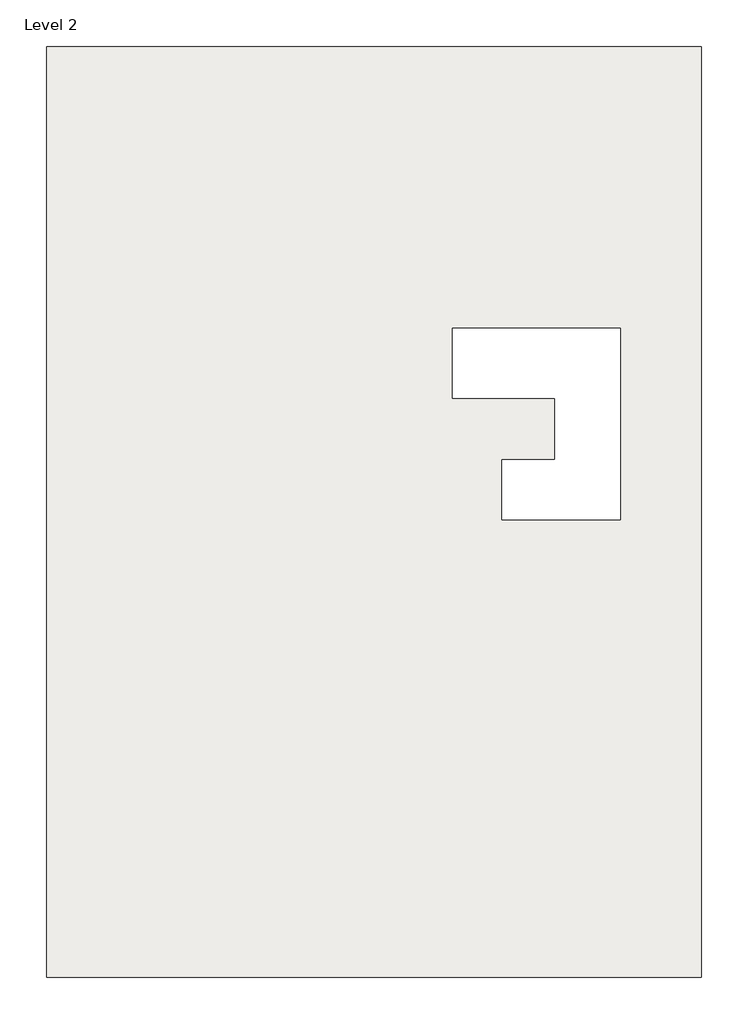
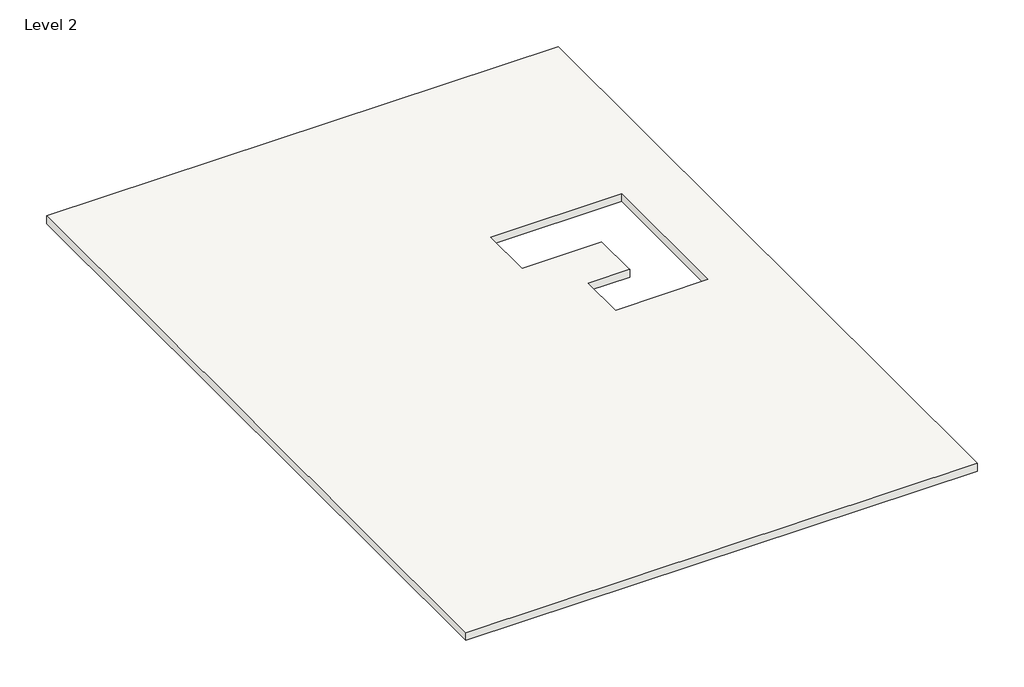
# One storey, incomplete: 1 roof.
"""IFC4 building model written with IfcOpenShell, lengths in millimetres."""

from ifc_helpers import new_model, si_unit, frame, origin, place, context, project, spatial, polyline, outline, extrude, element, save

model = new_model("IFC4")

# Units and contexts
model_context = context("Model", 3, world=origin())
ifc_project = project(units=[si_unit("LENGTHUNIT", "METRE", prefix="MILLI")], contexts=[model_context])

# Site, building, storey
site = spatial("IfcSite", under=ifc_project)
building = spatial("IfcBuilding", under=site)
storey = spatial("IfcBuildingStorey", under=building, Name="Level 2", Elevation=3048.0)

# Roof
placement = place(None, origin())
element("IfcRoof", 1, ObjectType="ROOF 6\"", at=placement, inside=storey, context=model_context, shape_type="SweptSolid", body=[
    extrude(outline(polyline([(-5513.0825206, 6650.5129493), (3910.3174794, 6650.5129493), (3910.3174794, -6735.2870507), (-5513.0825206, -6735.2870507), (-5513.0825206, 6650.5129493)]), holes=[polyline([(2741.9174794, -156.6870507), (2741.9174794, 2599.2129493), (328.9174794, 2599.2129493), (328.9174794, 1595.9129493), (1802.1174794, 1595.9129493), (1802.1174794, 706.9129493), (1040.1174794, 706.9129493), (1040.1174794, -156.6870507), (2741.9174794, -156.6870507)])]), frame((0.0, 0.0, 3048.0), z_axis=(0.0, 0.0, 1.0), x_axis=(1.0, 0.0, 0.0)), (0.0, 0.0, 1.0), 152.4),
])

save(model, "model.ifc")

# Revit data of these elements
# Type "ROOF 6\""
#   Assembly Code = "B1020"
#   Layers, outside or top first: 0' - 6" no material (function 1)
# Element 1 (IfcRoof, "ROOF 6\"")
#   built-in parameter 1001705 = 10.5 (stored number, unit not read)
#   built-in parameter 1001710 = 33615
#   Phase Created = New Construction
#   Materials on its faces: "Default Roof", "Birch"
# Materials
#   "Default Roof": colour RGB 88 101 114, transparency 0, Cost = 0
#   "Birch": class "Wood", colour RGB 224 178 126, transparency 0, Description = "Betula Alleghaniensis", Cost = 0
